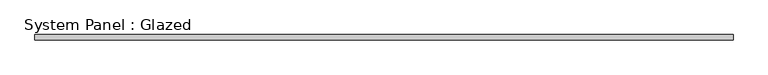
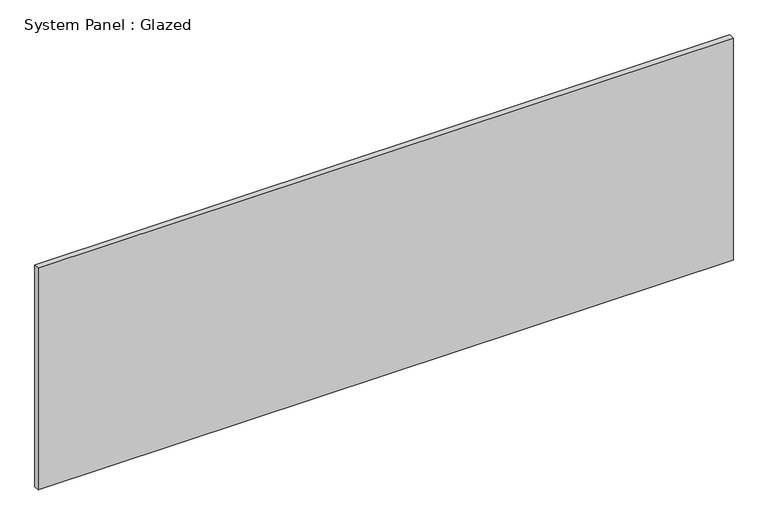
"""IFC4 building model written with IfcOpenShell, lengths in millimetres: plate geometry, System Panel : Glazed."""

from ifc_helpers import new_model, si_unit, origin, origin_with_axes, place, context, project, spatial, polyline, outline, extrude, source, transform, mapped, element, save


def system_panel_glazed_8818662e(model_context):
    return source(origin(), model_context, "Body", "SweptSolid", [
        extrude(outline(polyline([(1616.075, 19.05), (-1616.075, 19.05), (-1616.075, 44.45), (1616.075, 44.45), (1616.075, 19.05)])), origin_with_axes(), (0.0, 0.0, 1.0), 1092.2),
    ])


if __name__ == "__main__":
    model = new_model("IFC4")
    model_context = context("Model", 3, world=origin())
    ifc_project = project(units=[si_unit("LENGTHUNIT", "METRE", prefix="MILLI")], contexts=[model_context])
    site = spatial("IfcSite", under=ifc_project)
    building = spatial("IfcBuilding", under=site)
    placement = place(None, origin())
    system_panel_glazed_shape = system_panel_glazed_8818662e(model_context)
    element("IfcPlate", 1, ObjectType="System Panel : Glazed", at=placement, inside=building, context=model_context, shape_type="MappedRepresentation", body=[
        mapped(system_panel_glazed_shape, transform((0.0, 0.0, 0.0), x_axis=(1.0, 0.0, 0.0), y_axis=(0.0, 1.0, 0.0), z_axis=(0.0, 0.0, 1.0))),
    ])
    save(model, "model.ifc")

# Revit data of these elements
# Type "System Panel : Glazed"
#   Construction Type Id = "GSP4R"
#   Analytic Construction = "1/8 in Pilkington single glazing"
#   Visual Light Transmittance = 0.9
#   Solar Heat Gain Coefficient = 0.86
#   Heat Transfer Coefficient (U) = 1.18115 BTU/(h·ft²·°F)
# Element 1 (IfcPlate, "System Panel : Glazed")
#   Materials on its faces: "Glass"
# Materials
#   "Glass": class "Glass", colour RGB 0 128 192, transparency 0.75, Description = "Soda Lime Glass", Cost = 0
